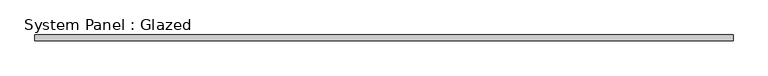
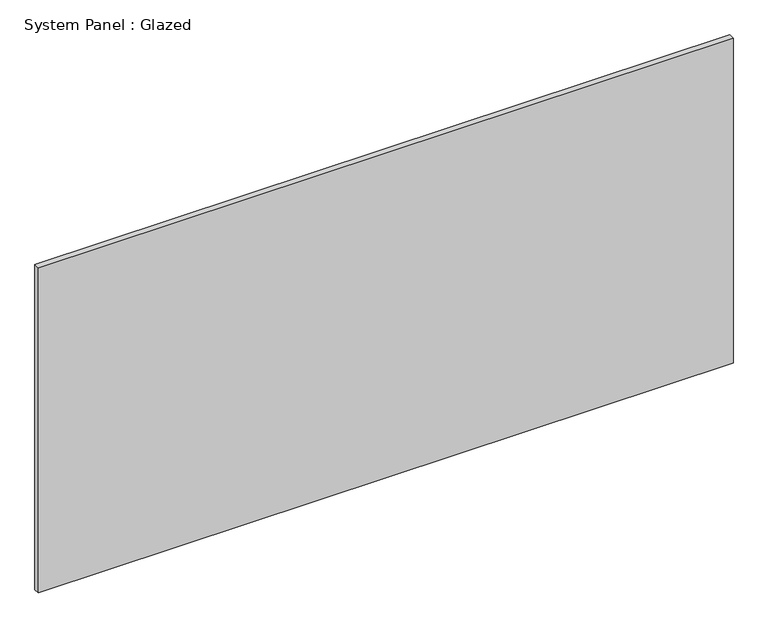
"""IFC4 building model written with IfcOpenShell, lengths in millimetres: plate geometry, System Panel : Glazed."""

from ifc_helpers import new_model, si_unit, origin, origin_with_axes, place, context, project, spatial, polyline, outline, extrude, source, transform, mapped, element, save


def system_panel_glazed_e46d4b42(model_context):
    return source(origin(), model_context, "Body", "SweptSolid", [
        extrude(outline(polyline([(1476.3750002, 19.05), (-1476.3750002, 19.05), (-1476.3750002, 44.45), (1476.3750002, 44.45), (1476.3750002, 19.05)])), origin_with_axes(), (0.0, 0.0, 1.0), 1460.5),
    ])


if __name__ == "__main__":
    model = new_model("IFC4")
    model_context = context("Model", 3, world=origin())
    ifc_project = project(units=[si_unit("LENGTHUNIT", "METRE", prefix="MILLI")], contexts=[model_context])
    site = spatial("IfcSite", under=ifc_project)
    building = spatial("IfcBuilding", under=site)
    placement = place(None, origin())
    system_panel_glazed_shape = system_panel_glazed_e46d4b42(model_context)
    element("IfcPlate", 1, ObjectType="System Panel : Glazed", at=placement, inside=building, context=model_context, shape_type="MappedRepresentation", body=[
        mapped(system_panel_glazed_shape, transform((0.0, 0.0, 0.0), x_axis=(1.0, 0.0, 0.0), y_axis=(0.0, 1.0, 0.0), z_axis=(0.0, 0.0, 1.0))),
    ])
    save(model, "model.ifc")

# Revit data of these elements
# Type "System Panel : Glazed"
#   Construction Type Id = "GSP4R"
#   Analytic Construction = "1/8 in Pilkington single glazing"
#   Visual Light Transmittance = 0.9
#   Solar Heat Gain Coefficient = 0.86
#   Heat Transfer Coefficient (U) = 1.18115 BTU/(h·ft²·°F)
#   Define Thermal Properties by = 1
# Element 1 (IfcPlate, "System Panel : Glazed")
#   Materials on its faces: "Glass"
# Materials
#   "Glass": class "Glass", colour RGB 0 128 192, transparency 0.75, Description = "Soda Lime Glass", Cost = 0
